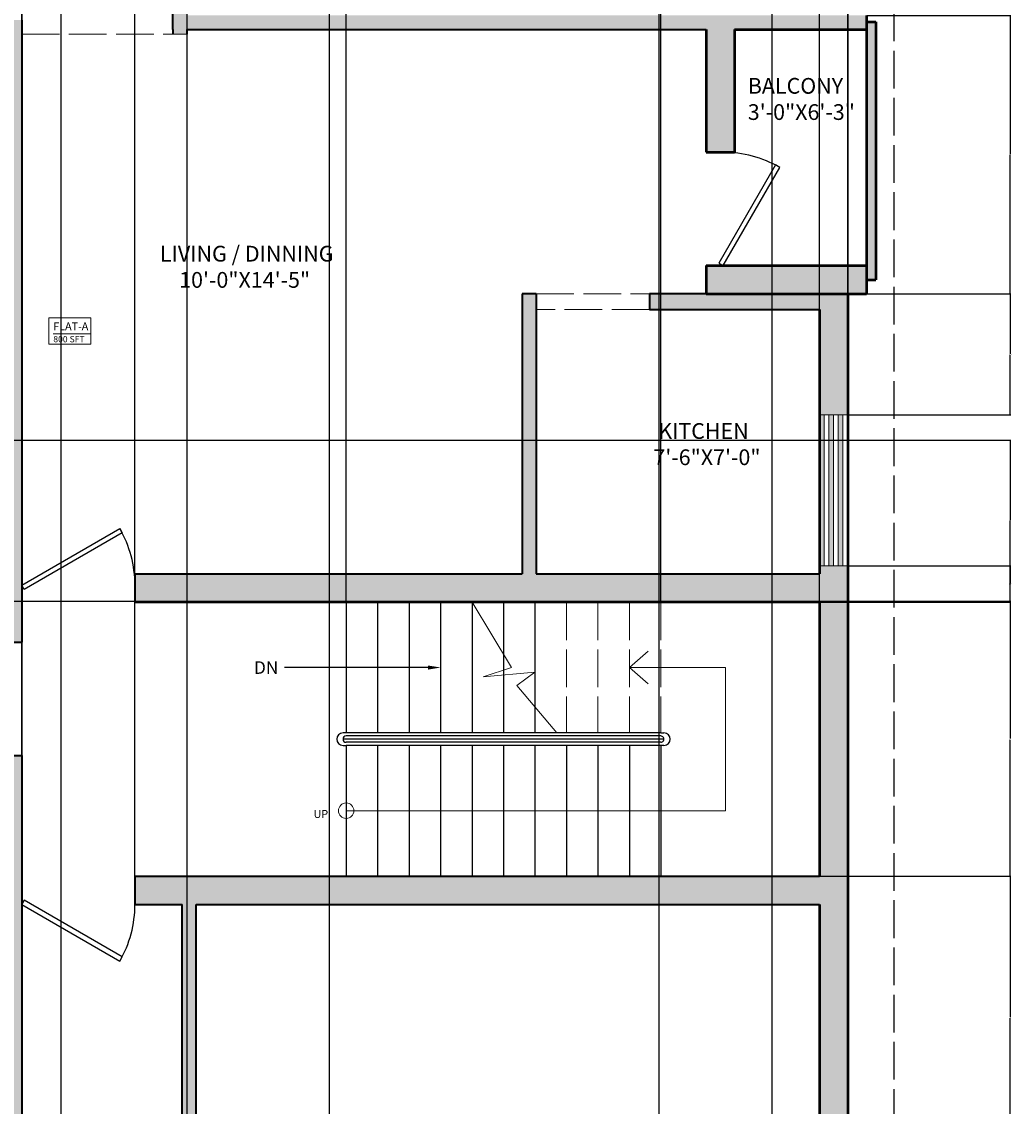
# Model space of a CAD drawing. Units: feet. Extents: x 2512 to 3087, y 1456 to 2266.
# Tile 4 of 5: x 2773 to 3087, y 1744 to 2088. Entities that reach past the tile are written whole.
import ezdxf
from ezdxf import colors
from ezdxf.entities.mleader import LeaderData, LeaderLine
from ezdxf.math import Vec2, Vec3

# ---------------------------------------------------------------- set-up
doc = ezdxf.new("R2010")
doc.units = ezdxf.units.FT
doc.linetypes.add('ACAD_ISO02W100', pattern=[15, 12, -3])
for name, color, linetype, lineweight in [('A-ANNO-DIMS', 2, 'Continuous', 18), ('A-ANNO-SYMB', 6, 'Continuous', 18), ('A-AREA-IDEN', 7, 'Continuous', 18), ('A-DOOR', 240, 'Continuous', 25), ('A-FLOR-STRS-OVHD', 6, 'ACAD_ISO02W100', 18), ('A-GLAZ', 4, 'Continuous', 18), ('A-WALL-PATT', 252, 'Continuous', 13), ('ANNOTATION', 80, 'Continuous', 18), ('C-PROP', 8, 'ACAD_ISO02W100', 25), ('INNER WALL', 7, 'Continuous', 35), ('OPEN DOOR', 50, 'ACAD_ISO02W100', 18), ('OUTER WALL', 7, 'Continuous', 50), ('STAIR', 6, 'Continuous', 25)]:
    doc.layers.add(name, color=color, linetype=linetype, lineweight=lineweight)
doc.styles.get("Standard").update_dxf_attribs({"font": 'arial.ttf'})
doc.dimstyles.get("Standard").update_dxf_attribs({"dimtxt": 0.18, "dimasz": 0.18, "dimexe": 0.18, "dimexo": 0.0625, "dimgap": 0.09, "dimtad": 0, "dimtih": 1, "dimtoh": 1, "dimdec": 4, "dimzin": 0, "dimdsep": 46, "dimtxsty": 'Standard', "dimcen": 0.09, "dimadec": 0, "dimazin": 0, "dimtfac": 1, "dimtdec": 4, "dimtofl": 0, "dimtmove": 0, "dimatfit": 3, "dimfxl": 1, "dimtolj": 1, "dimtzin": 0, "dimarcsym": 0})

# ---------------------------------------------------------------- blocks, each defined once
blk = doc.blocks.new('*U8')
for p, q in [((0, 0), (0, 6)), ((40, 0), (40, 6))]:
    blk.add_line(p, q)
blk.add_lwpolyline([(0, 0), (34.64, -20), (35.52, -18.48), (0.87, 1.52)], close=True)
blk.add_arc((0, 0), 40, 330, 0)
blk = doc.blocks.new('*U7')
for p, q in [((0, 0), (0, -6)), ((40, 0), (40, -6))]:
    blk.add_line(p, q)
blk.add_lwpolyline([(0, 0), (34.64, 20), (35.52, 18.48), (0.87, -1.52)], close=True)
blk.add_arc((0, 0), 40, 0, 30)
blk = doc.blocks.new('*U5')
for p, q in [((0, 0), (0, -6)), ((-40, 0), (-40, -6))]:
    blk.add_line(p, q)
blk.add_lwpolyline([(0, 0), (-34.64, 20), (-35.52, 18.48), (-0.88, -1.52)], close=True)
blk.add_arc((0, 0), 40, 150, 180)
blk = doc.blocks.new('WIN-48IN')
h = blk.add_hatch(color=256)
h.dxf.hatch_style = 1
h.paths.add_polyline_path([(0, 7.5), (0, 6), (48, 6), (48, 7.5)])
h.paths.add_polyline_path([(48, 3), (48, 4.5), (0, 4.5), (0, 3)])
h.paths.add_polyline_path([(48, 0), (48, 1.5), (0, 1.5), (0, 0)])
for p, q in [((0, 9), (48, 9)), ((0, 0), (0, 9)), ((0, 7.5), (48, 7.5)), ((48, 9), (48, 0)), ((0, 6), (48, 6)), ((0, 4.5), (48, 4.5)), ((0, 4.5), (48, 4.5)), ((0, 3), (48, 3)), ((0, 1.5), (48, 1.5)), ((48, 0), (0, 0))]:
    blk.add_line(p, q)
blk = doc.blocks.new('FLAT-ID-FRAME')
blk.add_line((1.44, 3.36), (13.18, 3.36))
blk.add_lwpolyline([(0, 8.39), (13.37, 8.39), (13.37, 0), (0, 0)], close=True)
blk = doc.blocks.new('*D23')
at = {"layer": 'A-ANNO-DIMS', "color": 0, "lineweight": -2, "transparency": 16777216}
for p, q in [((2772.72, 2204.17), (2772.72, 1456.05)), ((2785.14, 2204.17), (2785.14, 1456.05)), ((2772.9, 1456.23), (2778.48, 1456.23)), ((2784.96, 1456.23), (2779.38, 1456.23))]:
    blk.add_line(p, q, dxfattribs=at)
at = {"layer": 'A-ANNO-DIMS', "color": 0, "transparency": 16777216}
for points in [[(2772.9, 1456.26), (2772.9, 1456.2), (2772.72, 1456.23)], [(2784.96, 1456.26), (2784.96, 1456.2), (2785.14, 1456.23)]]:
    blk.add_solid(points, dxfattribs=at)
at = {"layer": 'Defpoints', "color": 0, "transparency": 16777216}
for p in [(2772.72, 2204.23), (2785.14, 2204.23), (2785.14, 1456.23)]:
    blk.add_point(p, dxfattribs=at)
at = {"layer": 'A-ANNO-DIMS', "color": 0, "transparency": 16777216, "insert": (2778.93, 1456.23), "char_height": 0.18, "attachment_point": 5}
blk.add_mtext('\\A1;12.422', dxfattribs=at)
blk = doc.blocks.new('*D24')
at = {"layer": 'A-ANNO-DIMS', "color": 0, "lineweight": -2, "transparency": 16777216}
for p, q in [((2825.22, 2204.17), (2825.22, 1456.05)), ((2870.39, 2204.17), (2870.39, 1456.05)), ((2825.4, 1456.23), (2847.41, 1456.23)), ((2870.21, 1456.23), (2848.2, 1456.23))]:
    blk.add_line(p, q, dxfattribs=at)
at = {"layer": 'A-ANNO-DIMS', "color": 0, "transparency": 16777216}
for points in [[(2825.4, 1456.26), (2825.4, 1456.2), (2825.22, 1456.23)], [(2870.21, 1456.26), (2870.21, 1456.2), (2870.39, 1456.23)]]:
    blk.add_solid(points, dxfattribs=at)
at = {"layer": 'Defpoints', "color": 0, "transparency": 16777216}
for p in [(2825.22, 2204.23), (2870.39, 2204.23), (2870.39, 1456.23)]:
    blk.add_point(p, dxfattribs=at)
at = {"layer": 'A-ANNO-DIMS', "color": 0, "transparency": 16777216, "insert": (2847.81, 1456.23), "char_height": 0.18, "attachment_point": 5}
blk.add_mtext('\\A1;45.17', dxfattribs=at)
blk = doc.blocks.new('*D37')
at = {"layer": 'A-ANNO-DIMS', "color": 0, "lineweight": -2, "transparency": 16777216}
for p, q in [((3026.28, 1816.73), (3087.03, 1816.73)), ((3086.85, 1816.55), (3086.85, 1771.91)), ((3086.85, 1726.91), (3086.85, 1771.55)), ((3035.28, 1726.73), (3087.03, 1726.73))]:
    blk.add_line(p, q, dxfattribs=at)
at = {"layer": 'A-ANNO-DIMS', "color": 0, "transparency": 16777216}
for points in [[(3086.82, 1816.55), (3086.88, 1816.55), (3086.85, 1816.73)], [(3086.82, 1726.91), (3086.88, 1726.91), (3086.85, 1726.73)]]:
    blk.add_solid(points, dxfattribs=at)
at = {"layer": 'Defpoints', "color": 0, "transparency": 16777216}
for p in [(3026.22, 1816.73), (3086.85, 1816.73), (3035.22, 1726.73)]:
    blk.add_point(p, dxfattribs=at)
at = {"layer": 'A-ANNO-DIMS', "color": 0, "transparency": 16777216, "insert": (3086.85, 1771.73), "char_height": 0.18, "attachment_point": 5}
blk.add_mtext('\\A1;90', dxfattribs=at)
blk = doc.blocks.new('*D38')
at = {"layer": 'A-ANNO-DIMS', "color": 0, "lineweight": -2, "transparency": 16777216}
for p, q in [((3026.28, 1903.73), (3087.03, 1903.73)), ((3086.85, 1903.55), (3086.85, 1860.41)), ((3086.85, 1816.91), (3086.85, 1860.05)), ((3026.28, 1816.73), (3087.03, 1816.73))]:
    blk.add_line(p, q, dxfattribs=at)
at = {"layer": 'A-ANNO-DIMS', "color": 0, "transparency": 16777216}
for points in [[(3086.82, 1903.55), (3086.88, 1903.55), (3086.85, 1903.73)], [(3086.82, 1816.91), (3086.88, 1816.91), (3086.85, 1816.73)]]:
    blk.add_solid(points, dxfattribs=at)
at = {"layer": 'Defpoints', "color": 0, "transparency": 16777216}
for p in [(3026.22, 1903.73), (3086.85, 1903.73), (3026.22, 1816.73)]:
    blk.add_point(p, dxfattribs=at)
at = {"layer": 'A-ANNO-DIMS', "color": 0, "transparency": 16777216, "insert": (3086.85, 1860.23), "char_height": 0.18, "attachment_point": 5}
blk.add_mtext('\\A1;87', dxfattribs=at)
blk = doc.blocks.new('*D39')
at = {"layer": 'A-ANNO-DIMS', "color": 0, "lineweight": -2, "transparency": 16777216}
for p, q in [((3035.28, 1915.29), (3087.03, 1915.29)), ((3086.85, 1915.11), (3086.85, 1909.69)), ((3086.85, 1903.91), (3086.85, 1909.33)), ((3026.28, 1903.73), (3087.03, 1903.73))]:
    blk.add_line(p, q, dxfattribs=at)
at = {"layer": 'A-ANNO-DIMS', "color": 0, "transparency": 16777216}
for points in [[(3086.82, 1915.11), (3086.88, 1915.11), (3086.85, 1915.29)], [(3086.82, 1903.91), (3086.88, 1903.91), (3086.85, 1903.73)]]:
    blk.add_solid(points, dxfattribs=at)
at = {"layer": 'Defpoints', "color": 0, "transparency": 16777216}
for p in [(3035.22, 1915.29), (3086.85, 1915.29), (3026.22, 1903.73)]:
    blk.add_point(p, dxfattribs=at)
at = {"layer": 'A-ANNO-DIMS', "color": 0, "transparency": 16777216, "insert": (3086.85, 1909.51), "char_height": 0.18, "attachment_point": 5}
blk.add_mtext('\\A1;11.556', dxfattribs=at)
blk = doc.blocks.new('*D40')
at = {"layer": 'A-ANNO-DIMS', "color": 0, "lineweight": -2, "transparency": 16777216}
for p, q in [((3035.28, 2001.73), (3087.03, 2001.73)), ((3086.85, 2001.55), (3086.85, 1982.69)), ((3086.85, 1963.47), (3086.85, 1982.33)), ((3035.28, 1963.29), (3087.03, 1963.29))]:
    blk.add_line(p, q, dxfattribs=at)
at = {"layer": 'A-ANNO-DIMS', "color": 0, "transparency": 16777216}
for points in [[(3086.82, 2001.55), (3086.88, 2001.55), (3086.85, 2001.73)], [(3086.82, 1963.47), (3086.88, 1963.47), (3086.85, 1963.29)]]:
    blk.add_solid(points, dxfattribs=at)
at = {"layer": 'Defpoints', "color": 0, "transparency": 16777216}
for p in [(3035.22, 2001.73), (3086.85, 2001.73), (3035.22, 1963.29)]:
    blk.add_point(p, dxfattribs=at)
at = {"layer": 'A-ANNO-DIMS', "color": 0, "transparency": 16777216, "insert": (3086.85, 1982.51), "char_height": 0.18, "attachment_point": 5}
blk.add_mtext('\\A1;38.444', dxfattribs=at)
blk = doc.blocks.new('*D41')
at = {"layer": 'A-ANNO-DIMS', "color": 0, "lineweight": -2, "transparency": 16777216}
for p, q in [((3041.28, 2090.23), (3087.03, 2090.23)), ((3086.85, 2090.05), (3086.85, 2046.16)), ((3086.85, 2001.91), (3086.85, 2045.8)), ((3041.28, 2001.73), (3087.03, 2001.73))]:
    blk.add_line(p, q, dxfattribs=at)
at = {"layer": 'A-ANNO-DIMS', "color": 0, "transparency": 16777216}
for points in [[(3086.82, 2090.05), (3086.88, 2090.05), (3086.85, 2090.23)], [(3086.82, 2001.91), (3086.88, 2001.91), (3086.85, 2001.73)]]:
    blk.add_solid(points, dxfattribs=at)
at = {"layer": 'Defpoints', "color": 0, "transparency": 16777216}
for p in [(3041.22, 2090.23), (3086.85, 2090.23), (3041.22, 2001.73)]:
    blk.add_point(p, dxfattribs=at)
at = {"layer": 'A-ANNO-DIMS', "color": 0, "transparency": 16777216, "insert": (3086.85, 2045.98), "char_height": 0.18, "attachment_point": 5}
blk.add_mtext('\\A1;88.5', dxfattribs=at)
blk = doc.blocks.new('*D44')
at = {"layer": 'A-ANNO-DIMS', "color": 0, "lineweight": -2, "transparency": 16777216}
for p, q in [((2975.22, 2135.17), (2975.22, 1456.05)), ((3035.22, 2135.17), (3035.22, 1456.05)), ((2975.4, 1456.23), (3005, 1456.23)), ((3035.04, 1456.23), (3005.44, 1456.23))]:
    blk.add_line(p, q, dxfattribs=at)
at = {"layer": 'A-ANNO-DIMS', "color": 0, "transparency": 16777216}
for points in [[(2975.4, 1456.26), (2975.4, 1456.2), (2975.22, 1456.23)], [(3035.04, 1456.26), (3035.04, 1456.2), (3035.22, 1456.23)]]:
    blk.add_solid(points, dxfattribs=at)
at = {"layer": 'Defpoints', "color": 0, "transparency": 16777216}
for p in [(2975.22, 2135.23), (3035.22, 2135.23), (3035.22, 1456.23)]:
    blk.add_point(p, dxfattribs=at)
at = {"layer": 'A-ANNO-DIMS', "color": 0, "transparency": 16777216, "insert": (3005.22, 1456.23), "char_height": 0.18, "attachment_point": 5}
blk.add_mtext('\\A1;60', dxfattribs=at)
blk = doc.blocks.new('*D45')
at = {"layer": 'A-ANNO-DIMS', "color": 0, "lineweight": -2, "transparency": 16777216}
for p, q in [((3011.22, 1678.79), (3011.22, 2266.2)), ((3011.4, 2266.02), (3023, 2266.02)), ((3035.04, 2266.02), (3023.44, 2266.02)), ((3035.22, 1678.79), (3035.22, 2266.2))]:
    blk.add_line(p, q, dxfattribs=at)
at = {"layer": 'A-ANNO-DIMS', "color": 0, "transparency": 16777216}
for points in [[(3011.4, 2266.05), (3011.4, 2265.99), (3011.22, 2266.02)], [(3035.04, 2266.05), (3035.04, 2265.99), (3035.22, 2266.02)]]:
    blk.add_solid(points, dxfattribs=at)
at = {"layer": 'Defpoints', "color": 0, "transparency": 16777216}
for p in [(3035.22, 2266.02), (3011.22, 1678.73), (3035.22, 1678.73)]:
    blk.add_point(p, dxfattribs=at)
at = {"layer": 'A-ANNO-DIMS', "color": 0, "transparency": 16777216, "insert": (3023.22, 2266.02), "char_height": 0.18, "attachment_point": 5}
blk.add_mtext('\\A1;24', dxfattribs=at)
blk = doc.blocks.new('*D46')
at = {"layer": 'A-ANNO-DIMS', "color": 0, "lineweight": -2, "transparency": 16777216}
for p, q in [((2573.28, 1955.22), (3087.03, 1955.22)), ((3086.85, 1955.04), (3086.85, 1929.84)), ((3086.85, 1904.28), (3086.85, 1929.47)), ((2573.28, 1904.1), (3087.03, 1904.1))]:
    blk.add_line(p, q, dxfattribs=at)
at = {"layer": 'A-ANNO-DIMS', "color": 0, "transparency": 16777216}
for points in [[(3086.82, 1955.04), (3086.88, 1955.04), (3086.85, 1955.22)], [(3086.82, 1904.28), (3086.88, 1904.28), (3086.85, 1904.1)]]:
    blk.add_solid(points, dxfattribs=at)
at = {"layer": 'Defpoints', "color": 0, "transparency": 16777216}
for p in [(2573.22, 1955.22), (2573.22, 1904.1), (3086.85, 1904.1)]:
    blk.add_point(p, dxfattribs=at)
at = {"layer": 'A-ANNO-DIMS', "color": 0, "transparency": 16777216, "insert": (3086.85, 1929.66), "char_height": 0.18, "attachment_point": 5}
blk.add_mtext('\\A1;51.12', dxfattribs=at)
blk = doc.blocks.new('*D50')
at = {"layer": 'A-ANNO-DIMS', "color": 0, "lineweight": -2, "transparency": 16777216}
for p, q in [((2875.84, 1903.79), (2875.84, 2266.2)), ((2876.02, 2266.02), (2925.56, 2266.02)), ((2975.66, 2266.02), (2926.12, 2266.02)), ((2975.84, 1903.79), (2975.84, 2266.2))]:
    blk.add_line(p, q, dxfattribs=at)
at = {"layer": 'A-ANNO-DIMS', "color": 0, "transparency": 16777216}
for points in [[(2876.02, 2266.05), (2876.02, 2265.99), (2875.84, 2266.02)], [(2975.66, 2266.05), (2975.66, 2265.99), (2975.84, 2266.02)]]:
    blk.add_solid(points, dxfattribs=at)
at = {"layer": 'Defpoints', "color": 0, "transparency": 16777216}
for p in [(2975.84, 2266.02), (2875.84, 1903.73), (2975.84, 1903.73)]:
    blk.add_point(p, dxfattribs=at)
at = {"layer": 'A-ANNO-DIMS', "color": 0, "transparency": 16777216, "insert": (2925.84, 2266.02), "char_height": 0.18, "attachment_point": 5}
blk.add_mtext('\\A1;100', dxfattribs=at)
blk = doc.blocks.new('*D51')
at = {"layer": 'A-ANNO-DIMS', "color": 0, "lineweight": -2, "transparency": 16777216}
for p, q in [((2975.84, 1903.79), (2975.84, 2266.2)), ((2976.02, 2266.02), (3000.63, 2266.02)), ((3026.04, 2266.02), (3001.42, 2266.02)), ((3026.22, 1903.79), (3026.22, 2266.2))]:
    blk.add_line(p, q, dxfattribs=at)
at = {"layer": 'A-ANNO-DIMS', "color": 0, "transparency": 16777216}
for points in [[(2976.02, 2266.05), (2976.02, 2265.99), (2975.84, 2266.02)], [(3026.04, 2266.05), (3026.04, 2265.99), (3026.22, 2266.02)]]:
    blk.add_solid(points, dxfattribs=at)
at = {"layer": 'Defpoints', "color": 0, "transparency": 16777216}
for p in [(3026.22, 2266.02), (2975.84, 1903.73), (3026.22, 1903.73)]:
    blk.add_point(p, dxfattribs=at)
at = {"layer": 'A-ANNO-DIMS', "color": 0, "transparency": 16777216, "insert": (3001.03, 2266.02), "char_height": 0.18, "attachment_point": 5}
blk.add_mtext('\\A1;50.38', dxfattribs=at)
blk = doc.blocks.new('*D52')
at = {"layer": 'A-ANNO-DIMS', "color": 0, "lineweight": -2, "transparency": 16777216}
for p, q in [((2772.72, 1813.15), (2772.72, 2266.2)), ((2772.9, 2266.02), (2790.5, 2266.02)), ((2808.54, 2266.02), (2790.94, 2266.02)), ((2808.72, 1816.79), (2808.72, 2266.2))]:
    blk.add_line(p, q, dxfattribs=at)
at = {"layer": 'A-ANNO-DIMS', "color": 0, "transparency": 16777216}
for points in [[(2772.9, 2266.05), (2772.9, 2265.99), (2772.72, 2266.02)], [(2808.54, 2266.05), (2808.54, 2265.99), (2808.72, 2266.02)]]:
    blk.add_solid(points, dxfattribs=at)
at = {"layer": 'Defpoints', "color": 0, "transparency": 16777216}
for p in [(2808.72, 2266.02), (2808.72, 1816.73), (2772.72, 1813.09)]:
    blk.add_point(p, dxfattribs=at)
at = {"layer": 'A-ANNO-DIMS', "color": 0, "transparency": 16777216, "insert": (2790.72, 2266.02), "char_height": 0.18, "attachment_point": 5}
blk.add_mtext('\\A1;36', dxfattribs=at)
blk = doc.blocks.new('*D54')
at = {"layer": 'A-ANNO-DIMS', "color": 0, "lineweight": -2, "transparency": 16777216}
for p, q in [((2772.72, 2132.17), (2772.72, 1456.05)), ((2763.72, 2127.67), (2763.72, 1456.05)), ((2763.9, 1456.23), (2768.07, 1456.23)), ((2772.54, 1456.23), (2768.37, 1456.23))]:
    blk.add_line(p, q, dxfattribs=at)
at = {"layer": 'A-ANNO-DIMS', "color": 0, "transparency": 16777216}
for points in [[(2763.9, 1456.26), (2763.9, 1456.2), (2763.72, 1456.23)], [(2772.54, 1456.26), (2772.54, 1456.2), (2772.72, 1456.23)]]:
    blk.add_solid(points, dxfattribs=at)
at = {"layer": 'Defpoints', "color": 0, "transparency": 16777216}
for p in [(2772.72, 2132.23), (2763.72, 2127.73), (2772.72, 1456.23)]:
    blk.add_point(p, dxfattribs=at)
at = {"layer": 'A-ANNO-DIMS', "color": 0, "transparency": 16777216, "insert": (2768.22, 1456.23), "char_height": 0.18, "attachment_point": 5}
blk.add_mtext('\\A1;9', dxfattribs=at)

msp = doc.modelspace()

# ---------------------------------------------------------------- hatches: boundary and pattern name
at = {"layer": 'A-WALL-PATT'}
h = msp.add_hatch(color=256, dxfattribs=at)
h.dxf.hatch_style = 1
h.paths.add_polyline_path([(3035.2185, 1915.2872), (3026.2185, 1915.2872), (3026.2185, 1912.7316), (2936.2185, 1912.7316), (2936.2185, 2001.7316), (2931.7185, 2001.7316), (2931.7185, 1912.7316), (2808.7185, 1912.7316), (2808.7185, 1903.7316), (3026.2185, 1903.7316), (3026.2185, 1816.7316), (2808.7185, 1816.7316), (2808.7185, 1807.7316), (2823.7185, 1807.7316), (2823.7185, 1638.2316), (2828.2185, 1638.2316), (2828.2185, 1674.2316), (2828.2185, 1678.7316), (2828.2185, 1807.7316), (3026.2185, 1807.7316), (3026.2185, 1735.7316), (3002.2185, 1735.7316), (3002.2546, 1726.7316), (3011.2546, 1726.7316), (3035.2185, 1726.7316)])
h.paths.add_polyline_path([(3035.2185, 2001.7316), (2990.2185, 2001.7316), (2972.2185, 2001.7316), (2972.2185, 1996.7316), (3026.2185, 1996.7316), (3026.2185, 1963.2872), (3035.2185, 1963.2872)], flags=17)
h.paths.add_polyline_path([(3041.2185, 2010.7316), (2990.2185, 2010.7316), (2990.2185, 2001.7316), (3035.2185, 2001.7316), (3041.2185, 2001.7316)])
h.paths.add_polyline_path([(3044.2185, 2085.7316), (3044.2185, 2088.2316), (3041.2185, 2088.2316), (3041.2185, 2006.2316), (3044.2185, 2006.2316)])
h.paths.add_polyline_path([(3041.2185, 2090.2316), (2975.2185, 2090.2316), (2975.2185, 2090.2254), (2966.2185, 2090.2254), (2825.2185, 2090.2316), (2825.2185, 2091.7316), (2820.7185, 2091.7316), (2820.7185, 2085.7316), (2820.7185, 2084.2316), (2825.2185, 2084.2316), (2825.2185, 2085.7316), (2990.2185, 2085.7316), (2990.2185, 2046.7316), (2999.2185, 2046.7316), (2999.2185, 2085.7316), (3041.2185, 2085.7316)])
h.paths.add_polyline_path([(3035.2185, 2213.2316), (2918.3922, 2213.2316), (2918.3922, 2204.2316), (3026.2185, 2204.2316), (3026.2185, 2144.2316), (2966.2185, 2144.2316), (2966.2185, 2135.213), (2975.2185, 2135.213), (2975.2185, 2135.2316), (3035.2185, 2135.2316)])
h.paths.add_polyline_path([(2870.3922, 2213.2316), (2809.1404, 2213.2316), (2809.1404, 2204.2316), (2820.7185, 2204.2316), (2820.7185, 2162.2316), (2825.2185, 2162.2316), (2825.2185, 2204.2316), (2870.3922, 2204.2316)])
h.paths.add_polyline_path([(2785.1404, 2213.2316), (2751.447, 2213.2316), (2751.447, 2204.2316), (2763.7185, 2204.2316), (2763.7185, 2127.7316), (2825.2185, 2127.7316), (2825.2185, 2132.2316), (2820.7185, 2132.2316), (2772.7185, 2132.2316), (2772.7185, 2204.2316), (2785.1404, 2204.2316)])
h.paths.add_polyline_path([(2727.447, 2213.2316), (2656.8898, 2213.2316), (2656.8898, 2204.2316), (2711.2185, 2204.2316), (2711.2185, 2124.7316), (2715.7185, 2124.7316), (2715.7185, 2127.7316), (2733.7185, 2127.7316), (2733.7185, 2132.2316), (2715.7185, 2132.2316), (2715.7185, 2204.2316), (2727.447, 2204.2316)], flags=17)
h.paths.add_polyline_path([(2608.8898, 2213.2316), (2564.2185, 2213.2316), (2564.2185, 2079.7316), (2609.2185, 2079.7316), (2609.2185, 2037.7316), (2618.2185, 2037.7316), (2618.2185, 2079.7316), (2763.7185, 2079.7316), (2763.7185, 2007.7316), (2654.2185, 2007.7316), (2654.2185, 2003.2316), (2763.7185, 2003.2316), (2763.7185, 1891.0755), (2772.7185, 1891.0234), (2772.7185, 1903.7316), (2772.7185, 2088.7316), (2573.2185, 2088.7316), (2573.2185, 2204.2316), (2608.8898, 2204.2316)])
h.paths.add_polyline_path([(2567.2185, 2079.7316), (2564.2185, 2079.7316), (2564.2185, 2007.7316), (2567.2185, 2007.7316)], flags=17)
h.paths.add_polyline_path([(2618.2185, 2007.7316), (2564.2185, 2007.7316), (2564.2185, 2003.2171), (2573.2185, 2003.2171), (2573.2185, 2003.2316), (2618.2185, 2003.2316)], flags=17)
h.paths.add_polyline_path([(2573.2185, 1955.2171), (2564.2185, 1955.2171), (2564.2185, 1904.096), (2573.2185, 1904.096)], flags=17)
h.paths.add_polyline_path([(2573.2185, 1851.677), (2603.2185, 1851.5035), (2603.2195, 1856.0035), (2573.2185, 1856.1771), (2573.2185, 1856.096), (2564.2185, 1856.096), (2564.2185, 1785.728), (2594.2185, 1785.5544), (2600.2185, 1785.5197), (2637.7185, 1785.3028), (2637.7185, 1855.8039), (2633.2185, 1855.83), (2633.2185, 1789.8289), (2573.2185, 1790.176)])
h.paths.add_polyline_path([(2772.7185, 1855.0228), (2767.3185, 1855.0228), (2767.3004, 1855.0542), (2673.7185, 1855.5956), (2673.7185, 1851.0956), (2763.7185, 1850.575), (2763.7185, 1743.5732), (2564.2185, 1744.7273), (2564.2185, 1719.3702), (2573.2185, 1719.3702), (2573.2185, 1735.6751), (2633.2185, 1735.328), (2633.2185, 1717.3272), (2637.7185, 1717.3272), (2637.7185, 1735.302), (2772.7185, 1734.521)])
h.paths.add_polyline_path([(2697.7185, 1734.9549), (2693.2185, 1734.9809), (2693.2185, 1602.8011), (2697.7185, 1602.8011)])
h.paths.add_polyline_path([(2823.7185, 1561.2231), (2733.7185, 1561.7437), (2733.7185, 1552.7436), (2823.7185, 1552.2229)])
h.paths.add_polyline_path([(2697.7185, 1566.8011), (2693.2185, 1566.8011), (2693.2185, 1562.8011), (2682.4194, 1562.8011), (2682.4194, 1553.8011), (2693.2185, 1553.8011), (2693.2185, 1495.2316), (2697.7185, 1495.2316)])
h.paths.add_polyline_path([(2828.2185, 1495.2316), (2693.2185, 1495.2316), (2693.2185, 1493.2316), (2828.2185, 1493.2316)])
h.paths.add_polyline_path([(2828.2185, 1602.2316), (2823.7185, 1602.2316), (2823.7185, 1495.2316), (2828.2185, 1495.2316)])
h.paths.add_polyline_path([(3035.2185, 1523.0765), (3026.2185, 1523.0765), (3026.2185, 1513.7316), (2828.2185, 1513.7316), (2828.2185, 1504.7316), (3035.2185, 1504.7316)])
h.paths.add_polyline_path([(3026.2185, 1602.2316), (2906.2185, 1602.2316), (2906.2185, 1644.2316), (2901.7185, 1644.2316), (2901.7185, 1597.7316), (3026.2185, 1597.7316)])
h.paths.add_polyline_path([(3035.2185, 1678.7316), (2864.2185, 1678.7316), (2864.2185, 1674.2316), (3026.2185, 1674.2316), (3026.2185, 1642.5123), (3035.2185, 1642.5123)], flags=17)
h.paths.add_polyline_path([(3035.2185, 1618.5123), (3026.2185, 1618.5123), (3026.2185, 1571.0765), (3035.2185, 1571.0765)])
h = msp.add_hatch(color=256, dxfattribs=at)
h.dxf.hatch_style = 1
h.paths.add_polyline_path([(2573.2185, 2204.2316), (2608.8898, 2204.2316), (2608.8898, 2213.2316), (2564.2185, 2213.2316), (2564.2185, 2079.7316), (2609.2185, 2079.7316), (2609.2185, 2037.7316), (2613.7185, 2037.7316), (2618.2185, 2037.7316), (2618.2185, 2079.7316), (2763.7185, 2079.7316), (2763.7185, 2007.7316), (2654.2185, 2007.7316), (2654.2185, 2003.2316), (2763.7185, 2003.2316), (2763.7185, 1891.0755), (2772.7185, 1891.0234), (2772.7185, 1903.7316), (2772.7185, 2088.7316), (2573.2185, 2088.7316)])
h.paths.add_polyline_path([(2727.447, 2213.2316), (2656.8898, 2213.2316), (2656.8898, 2204.2316), (2711.2185, 2204.2316), (2711.2185, 2124.7316), (2715.7185, 2124.7316), (2715.7185, 2127.7316), (2733.7185, 2127.7316), (2733.7185, 2132.2316), (2715.7185, 2132.2316), (2715.7185, 2204.2316), (2727.447, 2204.2316)], flags=17)
h.paths.add_polyline_path([(2785.1404, 2213.2316), (2751.447, 2213.2316), (2751.447, 2204.2316), (2763.7185, 2204.2316), (2763.7185, 2127.7316), (2825.2185, 2127.7316), (2825.2185, 2132.2316), (2820.7185, 2132.2316), (2772.7185, 2132.2316), (2772.7185, 2204.2316), (2785.1404, 2204.2316)])
h.paths.add_polyline_path([(2966.2185, 2204.2316), (2825.2185, 2204.2316), (2825.2185, 2162.2316), (2820.7185, 2162.2316, 0.12053744), (2806.8695, 2158.8438), (2822.234, 2132.2316), (2825.2185, 2132.2316), (2825.2185, 2127.7316), (2826.1185, 2127.7316, -0.12053744), (2842.7373, 2123.6662), (2842.7545, 2123.696), (2844.1185, 2122.9085), (2826.1185, 2091.7316), (2825.2185, 2091.7316), (2825.2185, 2090.2316), (2966.2185, 2090.2316), (2966.2185, 2135.213), (2966.2185, 2144.2316)], flags=17)
h.paths.add_polyline_path([(2870.3922, 2213.2316), (2809.1404, 2213.2316), (2809.1404, 2204.2316), (2820.7185, 2204.2316), (2820.7185, 2162.2316), (2825.2185, 2162.2316), (2825.2185, 2204.2316), (2870.3922, 2204.2316)])
h.paths.add_polyline_path([(3035.2185, 2213.2316), (2918.3922, 2213.2316), (2918.3922, 2204.2316), (3026.2185, 2204.2316), (3026.2185, 2144.2316), (2966.2185, 2144.2316), (2966.2185, 2135.213), (2975.2185, 2135.213), (2975.2185, 2135.2316), (3035.2185, 2135.2316)])
h.paths.add_polyline_path([(2999.2185, 2085.7316), (3041.2185, 2085.7316), (3041.2185, 2090.2316), (2975.2185, 2090.2316), (2975.2185, 2090.2254), (2966.2185, 2090.2254), (2825.2185, 2090.2316), (2825.2185, 2091.7316), (2820.7185, 2091.7316), (2820.7185, 2085.7316), (2820.7185, 2084.2316), (2825.2185, 2084.2316), (2825.2185, 2085.7316), (2990.2185, 2085.7316), (2990.2185, 2046.7316), (2995.6185, 2046.7316), (2999.2185, 2046.7316)])
h.paths.add_polyline_path([(3041.2185, 2010.7316), (2990.2185, 2010.7316), (2990.2185, 2001.7316), (3041.2185, 2001.7316)])
h.paths.add_polyline_path([(3035.2185, 2001.7316), (2990.2185, 2001.7316), (2972.2185, 2001.7316), (2972.2185, 1996.7316), (3026.2185, 1996.7316), (3026.2185, 1963.2872), (3035.2185, 1963.2872)])
h.paths.add_polyline_path([(3044.2185, 2085.7316), (3044.2185, 2088.2316), (3041.2185, 2088.2316), (3041.2185, 2085.7316), (3041.2185, 2006.2316), (3044.2185, 2006.2316)])
h.paths.add_polyline_path([(2966.2185, 2135.213), (2966.2185, 2144.2316), (2966.2185, 2204.2316), (2918.3922, 2204.2316), (2825.2185, 2204.2316), (2825.2185, 2162.2316), (2820.7185, 2162.2316, 0.12053744), (2806.8695, 2158.8438), (2822.234, 2132.2316), (2825.2185, 2132.2316), (2825.2185, 2127.7316), (2826.1185, 2127.7316, -0.12053744), (2842.7373, 2123.6662), (2842.7545, 2123.696), (2844.1185, 2122.9085), (2826.1185, 2091.7316), (2825.2185, 2091.7316), (2825.2185, 2090.2316), (2966.2185, 2090.2316)], flags=17)
h.paths.add_polyline_path([(2869.2463, 2140.1407), (2910.0273, 2140.1407), (2910.0273, 2158.8321), (2869.2463, 2158.8321)], flags=8)
h = msp.add_hatch(color=256, dxfattribs=at)
h.dxf.hatch_style = 1
h.paths.add_polyline_path([(2573.2185, 1683.1742), (2637.6925, 1682.8012), (2637.6947, 1687.3013), (2573.2185, 1687.6743), (2573.2185, 1695.3702), (2564.2185, 1695.3702), (2564.2185, 1517.8011), (2624.2185, 1517.8011), (2633.2185, 1517.8011), (2633.2185, 1553.8011), (2634.4194, 1553.8011), (2634.4194, 1562.8011), (2624.2185, 1562.8011), (2624.2185, 1526.8011), (2573.2185, 1526.8011)])
h.paths.add_polyline_path([(2573.2185, 1735.6751), (2633.2185, 1735.328), (2633.2185, 1717.3272), (2637.7096, 1717.3272), (2637.7185, 1735.302), (2772.7185, 1734.521), (2772.7185, 1855.0228), (2673.7185, 1855.5956), (2673.7185, 1851.0956), (2763.7185, 1850.575), (2763.7185, 1743.5732), (2564.2185, 1744.7273), (2564.2185, 1719.3702), (2573.2185, 1719.3702)])
h.paths.add_polyline_path([(2828.2185, 1807.7316), (3026.2185, 1807.7316), (3026.2185, 1735.7316), (3002.2185, 1735.7316), (3002.2546, 1726.7316), (3011.2546, 1726.7316), (3035.2185, 1726.7316), (3035.2185, 1915.2872), (3026.2185, 1915.2872), (3026.2185, 1912.7316), (2936.2185, 1912.7316), (2936.2185, 2001.7316), (2931.7185, 2001.7316), (2931.7185, 1912.7316), (2808.7185, 1912.7316), (2808.7185, 1903.7316), (3026.2185, 1903.7316), (3026.2185, 1816.7316), (2808.7185, 1816.7316), (2808.7185, 1807.7316), (2823.7185, 1807.7316), (2823.7185, 1638.2316), (2828.2185, 1638.2316), (2828.2185, 1674.2316), (2828.2185, 1678.7316)])
h.paths.add_polyline_path([(3035.2185, 1678.7316), (2864.2185, 1678.7316), (2864.2185, 1674.2316), (3026.2185, 1674.2316), (3026.2185, 1642.5123), (3035.2185, 1642.5123)], flags=17)
h.paths.add_polyline_path([(3035.2185, 1618.5123), (3026.2185, 1618.5123), (3026.2185, 1571.0765), (3035.2185, 1571.0765)])
h.paths.add_polyline_path([(3026.2185, 1602.2316), (2906.2185, 1602.2316), (2906.2185, 1644.2316), (2901.7185, 1644.2316), (2901.7185, 1597.7316), (3026.2185, 1597.7316)])
h.paths.add_polyline_path([(3035.2185, 1523.0765), (3026.2185, 1523.0765), (3026.2185, 1513.7316), (2828.2185, 1513.7316), (2828.2185, 1504.7316), (3035.2185, 1504.7316)])
h.paths.add_polyline_path([(2828.2185, 1495.2316), (2693.2185, 1495.2316), (2693.2185, 1493.2316), (2828.2185, 1493.2316)])
h.paths.add_polyline_path([(2828.2185, 1602.2316), (2823.7185, 1602.2316), (2823.7185, 1495.2316), (2828.2185, 1495.2316)])
h.paths.add_polyline_path([(2823.7185, 1561.2231), (2733.7185, 1561.7437), (2733.7185, 1552.7436), (2823.7185, 1552.2229)])
h.paths.add_polyline_path([(2697.7185, 1566.8011), (2693.2185, 1566.8011), (2693.2185, 1562.8011), (2682.4194, 1562.8011), (2682.4194, 1553.8011), (2693.2185, 1553.8011), (2693.2185, 1495.2316), (2697.7185, 1495.2316)])
h.paths.add_polyline_path([(2697.7185, 1734.9549), (2693.2185, 1734.9809), (2693.2185, 1602.8011), (2697.7185, 1602.8011)])
h.paths.add_polyline_path([(2573.2185, 1851.677), (2603.2185, 1851.5035), (2603.2195, 1856.0035), (2573.2185, 1856.1771), (2573.2185, 1856.096), (2564.2185, 1856.096), (2564.2185, 1785.728), (2594.2185, 1785.5544), (2600.2185, 1785.5197), (2637.7185, 1785.3028), (2637.7185, 1855.8039), (2633.2185, 1855.83), (2633.2185, 1789.8289), (2573.2185, 1790.176)])
h.paths.add_polyline_path([(2573.2185, 1955.2171), (2564.2185, 1955.2171), (2564.2185, 1904.096), (2573.2185, 1904.096)])
h.paths.add_polyline_path([(2618.2185, 2007.7316), (2564.2185, 2007.7316), (2564.2185, 2003.2171), (2573.2185, 2003.2171), (2573.2185, 2003.2316), (2618.2185, 2003.2316)])
h.paths.add_polyline_path([(2567.2185, 2079.7316), (2564.2185, 2079.7316), (2564.2185, 2007.7316), (2567.2185, 2007.7316)])

# ---------------------------------------------------------------- linework, layer by layer
at = {"layer": 'A-ANNO-SYMB'}
for p, q in [((2915.8387, 1903.7316), (2928.3428, 1882.9816)), ((2965.8387, 1882.9816), (2971.8448, 1888.169)), ((2928.3428, 1882.9816), (2919.3443, 1879.983)), ((2996.4076, 1882.9816), (2965.8387, 1882.9816)), ((2965.8387, 1882.9816), (2971.8448, 1877.7943)), ((2996.4076, 1837.4816), (2996.4076, 1882.9816)), ((2919.3443, 1879.983), (2935.8387, 1881.5662)), ((2935.8387, 1881.5662), (2930.0453, 1877.2667)), ((2930.0453, 1877.2667), (2942.7371, 1862.2316)), ((2875.8387, 1837.4816), (2996.4076, 1837.4816))]:
    msp.add_line(p, q, dxfattribs=at)
msp.add_circle((2875.8387, 1837.4816), 2.455, dxfattribs=at)
at = {"layer": 'A-FLOR-STRS-OVHD'}
for p, q in [((2945.8387, 1903.7316), (2945.8387, 1862.2316)), ((2955.8387, 1903.7316), (2955.8387, 1862.2316)), ((2965.8387, 1903.7316), (2965.8387, 1862.2316)), ((2975.8387, 1903.7316), (2975.8387, 1862.2316))]:
    msp.add_line(p, q, dxfattribs=at)
at = {"layer": 'C-PROP'}
msp.add_line((3049.8469, 2229.0217), (3049.8469, 1493.2316), dxfattribs=at)
at = {"layer": 'INNER WALL'}
for p, q in [((2820.7185, 2085.7316), (2820.7185, 2091.7316)), ((2772.7185, 2088.7316), (2772.7185, 1903.7316)), ((2820.7185, 2085.7316), (2820.7185, 2084.2316)), ((2825.2185, 2085.7316), (2966.2185, 2085.7316)), ((2825.2185, 2085.7316), (2990.2185, 2085.7316)), ((2825.2185, 2085.7316), (2825.2185, 2084.2316)), ((2931.7185, 2001.7316), (2931.7185, 1912.7316)), ((2936.2185, 2001.7316), (2931.7185, 2001.7316)), ((2936.2185, 2001.7316), (2936.2185, 1912.7316)), ((2990.2185, 2001.7316), (2972.2185, 2001.7316)), ((2972.2185, 2001.7316), (2972.2185, 1996.7316)), ((2972.2185, 1996.7316), (3026.2185, 1996.7316)), ((2808.7185, 1912.7316), (2931.7185, 1912.7316)), ((2808.7185, 1912.7316), (2808.7185, 1903.7316)), ((2936.2185, 1912.7316), (3026.2185, 1912.7316)), ((2772.7185, 1903.7316), (2772.7185, 1891.0234)), ((2808.7185, 1903.7316), (3026.2185, 1903.7316)), ((2763.7185, 1891.0755), (2772.9268, 1891.0222)), ((2673.7185, 1855.5956), (2772.7185, 1855.0228)), ((2772.7185, 1855.0228), (2772.7185, 1734.521)), ((2808.7185, 1816.7316), (3026.2185, 1816.7316)), ((2808.7185, 1816.7316), (2808.7185, 1807.7316)), ((2808.7185, 1807.7316), (2823.7185, 1807.7316)), ((2823.7185, 1638.2316), (2823.7185, 1807.7316)), ((2828.2185, 1807.7316), (3026.2185, 1807.7316)), ((2828.2185, 1678.7316), (2828.2185, 1807.7316))]:
    msp.add_line(p, q, dxfattribs=at)
at = {"layer": 'OPEN DOOR'}
for p, q in [((2772.7185, 2084.2316), (2825.2185, 2084.2316)), ((2936.2185, 2001.7316), (2972.2185, 2001.7316)), ((2972.2185, 1996.7316), (2936.2185, 1996.7316))]:
    msp.add_line(p, q, dxfattribs=at)
at = {"layer": 'OUTER WALL'}
for p, q in [((3041.2185, 2090.2316), (3041.2185, 2001.7316)), ((2990.2185, 2085.7316), (2990.2185, 2046.7316)), ((2999.2185, 2085.7316), (2999.2185, 2046.7316)), ((2999.2185, 2085.7316), (3041.2185, 2085.7316)), ((3041.2185, 2088.2316), (3044.2185, 2088.2316)), ((3044.2185, 2088.2316), (3044.2185, 2085.7316)), ((3044.2185, 2085.7316), (3044.2185, 2006.2316)), ((2990.2185, 2046.7316), (2999.2185, 2046.7316)), ((2990.2185, 2010.7316), (3041.2185, 2010.7316)), ((2990.2185, 2010.7316), (2990.2185, 2001.7316)), ((3041.2185, 2006.2316), (3044.2185, 2006.2316)), ((2990.2185, 2001.7316), (3041.2185, 2001.7316)), ((3035.2185, 2001.7316), (3035.2185, 1726.7316)), ((3026.2185, 1996.7316), (3026.2185, 1912.7316)), ((3026.2185, 1903.7316), (3026.2185, 1816.7316)), ((3026.2185, 1807.7316), (3026.2185, 1735.7316))]:
    msp.add_line(p, q, dxfattribs=at)
at = {"layer": 'STAIR'}
for p, q in [((2875.8387, 1903.7316), (2875.8387, 1862.2316)), ((2885.8387, 1903.7316), (2885.8387, 1862.2316)), ((2895.8387, 1903.7316), (2895.8387, 1862.2316)), ((2905.8387, 1903.7316), (2905.8387, 1862.2316)), ((2915.8387, 1903.7316), (2915.8387, 1862.2316)), ((2925.8387, 1903.7316), (2925.8387, 1862.2316)), ((2935.8387, 1903.7316), (2935.8387, 1862.2316)), ((2875.8423, 1862.2316), (2874.8465, 1862.2316)), ((2975.8423, 1862.2316), (2875.8423, 1862.2316)), ((2975.8423, 1862.2316), (2976.831, 1862.2316)), ((2872.8465, 1860.2316), (2872.8465, 1860.2316)), ((2976.8256, 1860.2316), (2874.8423, 1860.2316)), ((2874.8465, 1858.2316), (2875.8423, 1858.2316)), ((2875.8387, 1858.2316), (2875.8387, 1816.7316)), ((2975.8423, 1861.2316), (2875.8423, 1861.2316)), ((2975.8423, 1859.2316), (2875.8423, 1859.2316)), ((2975.8423, 1858.2316), (2875.8423, 1858.2316)), ((2885.8387, 1858.2316), (2885.8387, 1816.7316)), ((2895.8387, 1858.2316), (2895.8387, 1816.7316)), ((2905.8387, 1858.2316), (2905.8387, 1816.7316)), ((2915.8387, 1858.2316), (2915.8387, 1816.7316)), ((2925.8387, 1858.2316), (2925.8387, 1816.7316)), ((2935.8387, 1858.2316), (2935.8387, 1816.7316)), ((2945.8387, 1858.2316), (2945.8387, 1816.7316)), ((2955.8387, 1858.2316), (2955.8387, 1816.7316)), ((2965.8387, 1858.2316), (2965.8387, 1816.7316)), ((2975.8387, 1858.2316), (2975.8387, 1816.7316)), ((2976.831, 1858.2316), (2975.8423, 1858.2316)), ((2978.831, 1860.2316), (2978.831, 1860.2316))]:
    msp.add_line(p, q, dxfattribs=at)
for centre, radius, start, end in [((2874.8465, 1860.2316), 2, 90, 180), ((2976.831, 1860.2316), 2, 0, 90), ((2874.8465, 1860.2316), 2, 180, 270), ((2875.8423, 1860.2316), 1, 90, 270), ((2975.8254, 1860.2316), 1.0001, 269.035061, 90.964939), ((2976.831, 1860.2316), 2, 270, 0)]:
    msp.add_arc(centre, radius, start, end, dxfattribs=at)

# ---------------------------------------------------------------- block references
at = {"layer": 'A-AREA-IDEN'}
msp.add_blockref('FLAT-ID-FRAME', (2781.33, 1985.721), dxfattribs=at)
at = {"layer": 'A-DOOR', "xscale": 0.9000000000000044, "yscale": 0.9000000000000044, "zscale": 0.9000000000000044, "rotation": 270}
msp.add_blockref('*U5', (2995.6185, 2010.7316), dxfattribs=at)
at = {"layer": 'A-DOOR', "xscale": 0.899999999999959, "yscale": 0.899999999999959, "zscale": 0.899999999999959}
for name, p in [('*U7', (2772.7185, 1909.1316)), ('*U8', (2772.7185, 1807.692))]:
    msp.add_blockref(name, p, dxfattribs=at)
at = {"layer": 'A-GLAZ', "rotation": 269.9999999999956}
msp.add_blockref('WIN-48IN', (3026.2189, 1963.287), dxfattribs=at)

# ---------------------------------------------------------------- texts
at = {"layer": 'A-ANNO-SYMB', "insert": (2865.4944, 1837.6959), "char_height": 2.5, "attachment_point": 1}
msp.add_mtext_dynamic_manual_height_columns('UP', width=6.608218, gutter_width=12.5, heights=[0], dxfattribs=at)
at = {"layer": 'A-AREA-IDEN', "attachment_point": 1}
for s, width, insert, char_height in [('FLAT-A', 12.525641, (2782.7717, 1992.6811), 2.5), ('800 SFT', 11.390914, (2782.7717, 1988.3386), 2)]:
    msp.add_mtext_dynamic_manual_height_columns(s, width=width, gutter_width=12.5, heights=[0], dxfattribs=dict(at, insert=insert, char_height=char_height))
at = {"layer": 'ANNOTATION', "char_height": 5, "attachment_point": 1}
for s, width, insert in [('\\A1;BALCONY\\P3\'-0"X6\'-3"', 34.832096, (3003.4739, 2070.3479)), ('\\A1;LIVING / DINNING\\P    10\'-0"X14\'-5"', 59.172495, (2816.6559, 2017.0047)), ('\\A1; KITCHEN\\P7\'-6"X7\'-0"', 38.558323, (2973.4742, 1960.6508))]:
    msp.add_mtext_dynamic_manual_height_columns(s, width=width, gutter_width=12.5, heights=[0], dxfattribs=dict(at, insert=insert))

# ---------------------------------------------------------------- dimensions: what is measured, and where the dimension line sits
at = {"layer": 'A-ANNO-DIMS'}
for base, p1, p2, override, picture, middle in [((2808.7185, 2266.0217), (2772.7185, 1813.092), (2808.7185, 1816.7316), {"dimdec": 0, "dimlfac": 1, "dimrnd": 0, "dimzin": 0, "dimdsep": 46, "dimlunit": 2}, '*D52', (2790.7185, 2266.0217)), ((2975.8387, 2266.0217), (2875.8387, 1903.7316), (2975.8387, 1903.7316), {"dimdec": 0, "dimlfac": 1, "dimrnd": 0, "dimzin": 0, "dimdsep": 46, "dimlunit": 2}, '*D50', (2925.8387, 2266.0217)), ((3026.2185, 2266.0217), (2975.8387, 1903.7316), (3026.2185, 1903.7316), {"dimdec": 2, "dimlfac": 1, "dimrnd": 0, "dimzin": 0, "dimdsep": 46, "dimlunit": 2}, '*D51', (3001.0286, 2266.0217)), ((3035.2185, 2266.0217), (3011.2185, 1678.7316), (3035.2185, 1678.7316), {"dimdec": 0, "dimlfac": 1, "dimrnd": 0, "dimzin": 0, "dimdsep": 46, "dimlunit": 2}, '*D45', (3023.2185, 2266.0217)), ((2785.1404, 1456.2316), (2772.7185, 2204.2316), (2785.1404, 2204.2316), {"dimdec": 3, "dimlfac": 1, "dimrnd": 0, "dimzin": 0, "dimdsep": 46, "dimlunit": 2}, '*D23', (2778.9294, 1456.2316)), ((2870.3922, 1456.2316), (2825.2185, 2204.2316), (2870.3922, 2204.2316), {"dimdec": 2, "dimlfac": 1, "dimrnd": 0, "dimzin": 0, "dimdsep": 46, "dimlunit": 2}, '*D24', (2847.8054, 1456.2316)), ((3035.2185, 1456.2316), (2975.2185, 2135.2316), (3035.2185, 2135.2316), {"dimdec": 0, "dimlfac": 1, "dimrnd": 0, "dimzin": 0, "dimdsep": 46, "dimlunit": 2}, '*D44', (3005.2185, 1456.2316)), ((2772.7185, 1456.2316), (2763.7185, 2127.7316), (2772.7185, 2132.2316), {"dimdec": 0, "dimlfac": 1, "dimrnd": 0, "dimzin": 0, "dimdsep": 46, "dimlunit": 2}, '*D54', (2768.2185, 1456.2316))]:
    dim = msp.add_linear_dim(base=base, p1=p1, p2=p2, dimstyle='Standard', override=override, dxfattribs=at)
    dim.commit()
    dim.dimension.update_dxf_attribs({"geometry": picture, "text_midpoint": middle})
for base, p1, p2, override, picture, middle in [((3086.8469, 2090.2316), (3041.2185, 2001.7316), (3041.2185, 2090.2316), {"dimdec": 1, "dimlfac": 1, "dimrnd": 0, "dimzin": 0, "dimdsep": 46, "dimlunit": 2}, '*D41', (3086.8469, 2045.9816)), ((3086.8469, 2001.7316), (3035.2185, 1963.2872), (3035.2185, 2001.7316), {"dimdec": 3, "dimlfac": 1, "dimrnd": 0, "dimzin": 0, "dimdsep": 46, "dimlunit": 2}, '*D40', (3086.8469, 1982.5094)), ((3086.8469, 1904.096), (2573.2185, 1955.2171), (2573.2185, 1904.096), {"dimdec": 2, "dimlfac": 1, "dimrnd": 0, "dimzin": 0, "dimdsep": 46, "dimlunit": 2}, '*D46', (3086.8469, 1929.6566)), ((3086.8469, 1915.2872), (3026.2185, 1903.7316), (3035.2185, 1915.2872), {"dimdec": 3, "dimlfac": 1, "dimrnd": 0, "dimzin": 0, "dimdsep": 46, "dimlunit": 2}, '*D39', (3086.8469, 1909.5094)), ((3086.8469, 1903.7316), (3026.2185, 1816.7316), (3026.2185, 1903.7316), {"dimdec": 0, "dimlfac": 1, "dimrnd": 0, "dimzin": 0, "dimdsep": 46, "dimlunit": 2}, '*D38', (3086.8469, 1860.2316)), ((3086.8469, 1816.7316), (3035.2185, 1726.7316), (3026.2185, 1816.7316), {"dimdec": 0, "dimlfac": 1, "dimrnd": 0, "dimzin": 0, "dimdsep": 46, "dimlunit": 2}, '*D37', (3086.8469, 1771.7316))]:
    dim = msp.add_linear_dim(base=base, p1=p1, p2=p2, angle=90, dimstyle='Standard', override=override, dxfattribs=at)
    dim.commit()
    dim.dimension.update_dxf_attribs({"geometry": picture, "text_midpoint": middle})

# ---------------------------------------------------------------- leaders
at = {"layer": 'A-ANNO-SYMB'}
ml = msp.add_multileader_mtext('Standard', dxfattribs=at)
ml.set_content('DN', color=256)
ml.set_leader_properties()
ml.build(insert=Vec2(0, 0))
ctx = ml.context
ctx.base_point, ctx.plane_origin = Vec3(2845.0818, 1882.9816), Vec3(2905.8387, 1882.9816)
ctx.text_align_type = 2
notes = []
notes.append((ctx, [(0, (1, 1, 0), (2864.2633, 1882.9816), (-1, 0), 8, [(0, [(2905.8387, 1882.9816)], 0, [])])]))
ctx.mtext.insert, ctx.mtext.alignment, ctx.mtext.flow_direction = Vec3(2854.2633, 1884.9816), 3, 5
for ctx, leaders in notes:
    for number, flags, end, landing, length, lines in leaders:
        leader = LeaderData()
        leader.index, (leader.has_last_leader_line, leader.has_dogleg_vector, leader.attachment_direction) = number, flags
        leader.last_leader_point, leader.dogleg_vector, leader.dogleg_length = Vec3(end), Vec3(landing), length
        for number, points, colour, breaks in lines:
            line = LeaderLine()
            line.index, line.vertices, line.color, line.breaks = number, Vec3.list(points), colors.encode_raw_color(colour), breaks
            leader.lines.append(line)
        ctx.leaders.append(leader)

doc.saveas('drawing.dxf')
